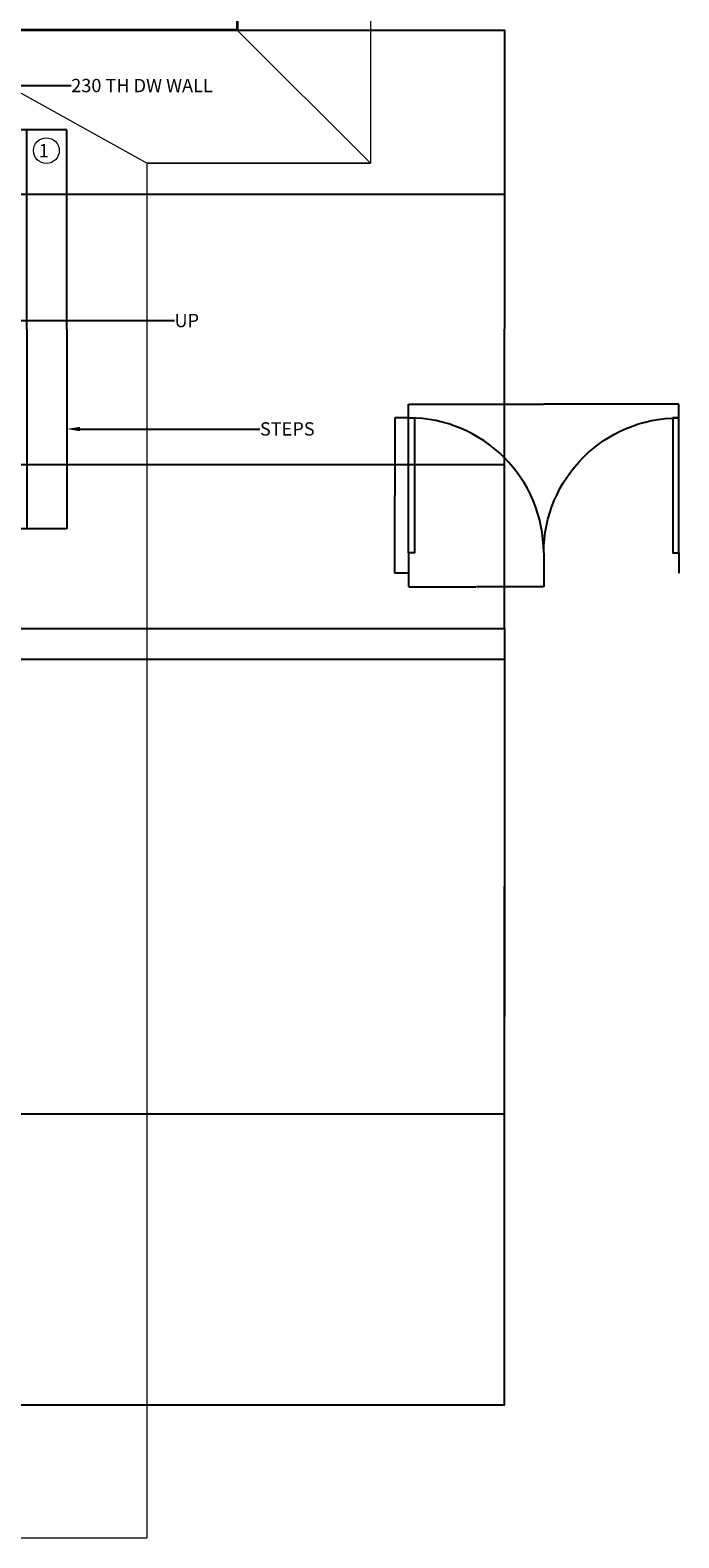
# Model space of a CAD drawing. Units: millimetres. Extents: x -8052 to 19968, y -37825 to -17505.
# Tile 9 of 10: x 10533 to 15409, y -36815 to -25475. Entities that reach past the tile are written whole.
import ezdxf
from ezdxf import colors
from ezdxf.entities.mleader import LeaderData, LeaderLine
from ezdxf.math import Vec2, Vec3

# ---------------------------------------------------------------- set-up
doc = ezdxf.new("R2010")
doc.units = ezdxf.units.MM
doc.header["$MEASUREMENT"] = 0
for name, color, linetype, lineweight in [('A-ANNO-DIMS', 2, 'Continuous', 18), ('A-ANNO-SYMB', 7, 'Continuous', 18), ('A-ANNO-TEXT', 7, 'Continuous', 18), ('A-DOOR', 3, 'Continuous', 25), ('A-FLOR', 8, 'Continuous', 18), ('A-FLOR-STRS', 7, 'Continuous', 25), ('A-WALL', 7, 'Continuous', 35)]:
    doc.layers.add(name, color=color, linetype=linetype, lineweight=lineweight)
doc.styles.get("Standard").update_dxf_attribs({"font": 'arial.ttf'})
doc.dimstyles.get("Standard").update_dxf_attribs({"dimtxt": 1.054, "dimasz": 1.055, "dimexe": 0.18, "dimexo": 0.0625, "dimgap": 0.09, "dimtad": 0, "dimtih": 1, "dimtoh": 1, "dimdec": 4, "dimzin": 0, "dimdsep": 46, "dimtxsty": 'Standard', "dimcen": 0.09, "dimadec": 0, "dimazin": 0, "dimtfac": 1, "dimtdec": 4, "dimtofl": 0, "dimtmove": 0, "dimatfit": 3, "dimfxl": 1, "dimtolj": 1, "dimtzin": 0, "dimarcsym": 0})

# ---------------------------------------------------------------- blocks, each defined once
blk = doc.blocks.new('*U21')
for p, q in [((0, 0), (0, -6)), ((40, 0), (40, -6))]:
    blk.add_line(p, q)
blk.add_lwpolyline([(0, 0), (0, 40), (1.75, 40), (1.75, 0)], close=True)
blk.add_arc((0, 0), 40, 0, 90)
blk = doc.blocks.new('STAIR-SIDE-ENTRY-3000')
for p, q in [((0, 1500), (0, 3000)), ((0, 3000), (1200, 3000)), ((300, 1500), (300, 3000)), ((300, 1500), (300, 3000)), ((600, 1500), (600, 3000)), ((900, 1500), (900, 3000)), ((0, 1500), (0, 1500)), ((0, 1500), (0, 0)), ((300, 1500), (300, 0)), ((600, 1500), (600, 0)), ((900, 1500), (900, 0)), ((0, 0), (1200, 0))]:
    blk.add_line(p, q)
blk = doc.blocks.new('*D97')
at = {"layer": 'A-ANNO-DIMS', "color": 0, "lineweight": -2, "transparency": 16777216}
for p, q in [((12090, -25475), (14100, -25475)), ((14099, -25476), (14099, -27724)), ((14099, -29974), (14099, -27725)), ((10410, -29975), (14100, -29975))]:
    blk.add_line(p, q, dxfattribs=at)
at = {"layer": 'A-ANNO-DIMS', "color": 0, "lineweight": 100, "transparency": 16777216}
for points in [[(14099, -25476), (14100, -25476), (14099, -25475)], [(14099, -29974), (14100, -29974), (14099, -29975)]]:
    blk.add_solid(points, dxfattribs=at)
at = {"layer": 'Defpoints', "color": 0, "lineweight": 100, "transparency": 16777216}
for p in [(12090, -25475), (10410, -29975), (14099, -29975)]:
    blk.add_point(p, dxfattribs=at)
at = {"layer": 'A-ANNO-DIMS', "color": 0, "transparency": 16777216, "insert": (14099, -27725), "char_height": 1.05, "attachment_point": 5}
blk.add_mtext('\\A1;4500', dxfattribs=at)
blk = doc.blocks.new('*D98')
at = {"layer": 'A-ANNO-DIMS', "color": 0, "lineweight": -2, "transparency": 16777216}
for p, q in [((10410, -29975), (14100, -29975)), ((14099, -29976), (14099, -32894)), ((14099, -35814), (14099, -32895)), ((10410, -35815), (14100, -35815))]:
    blk.add_line(p, q, dxfattribs=at)
at = {"layer": 'A-ANNO-DIMS', "color": 0, "lineweight": 100, "transparency": 16777216}
for points in [[(14099, -29976), (14100, -29976), (14099, -29975)], [(14099, -35814), (14100, -35814), (14099, -35815)]]:
    blk.add_solid(points, dxfattribs=at)
at = {"layer": 'Defpoints', "color": 0, "lineweight": 100, "transparency": 16777216}
for p in [(10410, -29975), (10410, -35815), (14099, -35815)]:
    blk.add_point(p, dxfattribs=at)
at = {"layer": 'A-ANNO-DIMS', "color": 0, "transparency": 16777216, "insert": (14099, -32895), "char_height": 1.05, "attachment_point": 5}
blk.add_mtext('\\A1;5840', dxfattribs=at)
blk = doc.blocks.new('*D109')
at = {"layer": 'A-ANNO-DIMS', "color": 0, "lineweight": -2, "transparency": 16777216}
for p, q in [((720, -30205), (14100, -30205)), ((14099, -30206), (14099, -31914)), ((14099, -33624), (14099, -31915)), ((950, -33625), (14100, -33625))]:
    blk.add_line(p, q, dxfattribs=at)
at = {"layer": 'A-ANNO-DIMS', "color": 0, "lineweight": 100, "transparency": 16777216}
for points in [[(14099, -30206), (14100, -30206), (14099, -30205)], [(14099, -33624), (14100, -33624), (14099, -33625)]]:
    blk.add_solid(points, dxfattribs=at)
at = {"layer": 'Defpoints', "color": 0, "lineweight": 100, "transparency": 16777216}
for p in [(720, -30205), (950, -33625), (14099, -33625)]:
    blk.add_point(p, dxfattribs=at)
at = {"layer": 'A-ANNO-DIMS', "color": 0, "transparency": 16777216, "insert": (14099, -31915), "char_height": 1.05, "attachment_point": 5}
blk.add_mtext('\\A1;3420', dxfattribs=at)
blk = doc.blocks.new('*D111')
at = {"layer": 'A-ANNO-DIMS', "color": 0, "lineweight": -2, "transparency": 16777216}
for p, q in [((-560, -26709), (14100, -26709)), ((14099, -26710), (14099, -27724)), ((14099, -28740), (14099, -27725)), ((-560, -28741), (14100, -28741))]:
    blk.add_line(p, q, dxfattribs=at)
at = {"layer": 'A-ANNO-DIMS', "color": 0, "lineweight": 100, "transparency": 16777216}
for points in [[(14099, -26710), (14100, -26710), (14099, -26709)], [(14099, -28740), (14100, -28740), (14099, -28741)]]:
    blk.add_solid(points, dxfattribs=at)
at = {"layer": 'Defpoints', "color": 0, "lineweight": 100, "transparency": 16777216}
for p in [(-560, -26709), (-560, -28741), (14099, -28741)]:
    blk.add_point(p, dxfattribs=at)
at = {"layer": 'A-ANNO-DIMS', "color": 0, "transparency": 16777216, "insert": (14099, -27725), "char_height": 1.05, "attachment_point": 5}
blk.add_mtext('\\A1;2032', dxfattribs=at)
blk = doc.blocks.new('*D126')
at = {"layer": 'A-ANNO-DIMS', "color": 0, "lineweight": -2, "transparency": 16777216}
for p, q in [((13377, -28391), (13377, -28288)), ((13378, -28289), (14391, -28289)), ((15408, -28289), (14395, -28289)), ((15409, -28391), (15409, -28288))]:
    blk.add_line(p, q, dxfattribs=at)
at = {"layer": 'A-ANNO-DIMS', "color": 0, "lineweight": 100, "transparency": 16777216}
for points in [[(13378, -28288), (13378, -28289), (13377, -28289)], [(15408, -28288), (15408, -28289), (15409, -28289)]]:
    blk.add_solid(points, dxfattribs=at)
at = {"layer": 'Defpoints', "color": 0, "lineweight": 100, "transparency": 16777216}
for p in [(15409, -28289), (13377, -28391), (15409, -28391)]:
    blk.add_point(p, dxfattribs=at)
at = {"layer": 'A-ANNO-DIMS', "color": 0, "transparency": 16777216, "insert": (14393, -28289), "char_height": 1.05, "attachment_point": 5}
blk.add_mtext('\\A1;2032', dxfattribs=at)
blk = doc.blocks.new('*D127')
at = {"layer": 'A-ANNO-DIMS', "color": 0, "lineweight": -2, "transparency": 16777216}
for p, q in [((13377, -28391), (13274, -28391)), ((13274, -28392), (13274, -28975)), ((13274, -29558), (13274, -28976)), ((13377, -29560), (13274, -29560))]:
    blk.add_line(p, q, dxfattribs=at)
at = {"layer": 'A-ANNO-DIMS', "color": 0, "lineweight": 100, "transparency": 16777216}
for points in [[(13274, -28392), (13275, -28392), (13274, -28391)], [(13274, -29558), (13275, -29558), (13274, -29560)]]:
    blk.add_solid(points, dxfattribs=at)
at = {"layer": 'Defpoints', "color": 0, "lineweight": 100, "transparency": 16777216}
for p in [(13274, -28391), (13377, -28391), (13377, -29560)]:
    blk.add_point(p, dxfattribs=at)
at = {"layer": 'A-ANNO-DIMS', "color": 0, "transparency": 16777216, "insert": (13274, -28975), "char_height": 1.05, "attachment_point": 5}
blk.add_mtext('\\A1;1168.4', dxfattribs=at)
blk = doc.blocks.new('*D128')
at = {"layer": 'A-ANNO-DIMS', "color": 0, "lineweight": -2, "transparency": 16777216}
for p, q in [((13377, -29407), (13377, -29662)), ((14393, -29407), (14393, -29662)), ((13378, -29662), (13883, -29662)), ((14392, -29662), (13887, -29662))]:
    blk.add_line(p, q, dxfattribs=at)
at = {"layer": 'A-ANNO-DIMS', "color": 0, "lineweight": 100, "transparency": 16777216}
for points in [[(13378, -29662), (13378, -29662), (13377, -29662)], [(14392, -29662), (14392, -29662), (14393, -29662)]]:
    blk.add_solid(points, dxfattribs=at)
at = {"layer": 'Defpoints', "color": 0, "lineweight": 100, "transparency": 16777216}
for p in [(13377, -29407), (14393, -29407), (14393, -29662)]:
    blk.add_point(p, dxfattribs=at)
at = {"layer": 'A-ANNO-DIMS', "color": 0, "transparency": 16777216, "insert": (13885, -29662), "char_height": 1.05, "attachment_point": 5}
blk.add_mtext('\\A1;1016', dxfattribs=at)

msp = doc.modelspace()

# ---------------------------------------------------------------- linework, layer by layer
at = {"layer": 'A-ANNO-SYMB'}
msp.add_circle((10654.35, -26381.051), 97, dxfattribs=at)
at = {"layer": 'A-FLOR'}
for p, q in [((13089.979, -18514.843), (13089.979, -26474.843)), ((11409.979, -26474.843), (9607.479, -25474.843)), ((12089.979, -25474.843), (13089.979, -26474.843)), ((11409.979, -26474.843), (11409.979, -36814.843)), ((13089.979, -26474.843), (11409.979, -26474.843)), ((13089.979, -26474.843), (11409.979, -26474.843)), ((11409.979, -26474.843), (13089.979, -26474.843)), ((11409.979, -26474.843), (11409.979, -36814.843)), ((-4710.021, -36814.843), (11409.979, -36814.843))]:
    msp.add_line(p, q, dxfattribs=at)
at = {"layer": 'A-WALL'}
for p, q in [((12089.979, -25244.843), (12089.979, -25474.843)), ((11859.979, -25474.843), (9359.979, -25474.843)), ((12089.979, -25474.843), (11859.979, -25474.843))]:
    msp.add_line(p, q, dxfattribs=at)

# ---------------------------------------------------------------- block references
at = {"layer": 'A-DOOR', "xscale": 25.39999999999996, "yscale": 25.39999999999996, "zscale": 25.39999999999996}
msp.add_blockref('*U21', (13376.928, -29407.126), dxfattribs=at)
at = {"layer": 'A-DOOR', "extrusion": (0, 0, -1), "xscale": 25.39999999999994, "yscale": 25.39999999999994, "zscale": -25.4}
msp.add_blockref('*U21', (-15408.928, -29407.126), dxfattribs=at)
at = {"layer": 'A-FLOR-STRS', "extrusion": (0, 0, -1), "zscale": -1}
msp.add_blockref('STAIR-SIDE-ENTRY-3000', (-10807.48, -29224.843), dxfattribs=at)

# ---------------------------------------------------------------- texts
at = {"layer": 'A-ANNO-TEXT', "insert": (10672.768, -26330.846), "char_height": 100, "attachment_point": 3}
msp.add_mtext_dynamic_manual_height_columns('1', width=159.07556, gutter_width=1, heights=[0], dxfattribs=at)

# ---------------------------------------------------------------- dimensions: what is measured, and where the dimension line sits
at = {"layer": 'A-ANNO-DIMS'}
for base, p1, p2, override, picture, middle in [((14099.479, -29974.843), (12089.979, -25474.843), (10409.979, -29974.843), {"dimdec": 0, "dimlfac": 1, "dimrnd": 0, "dimzin": 0, "dimdsep": 46, "dimlunit": 2}, '*D97', (14099.479, -27724.843)), ((14099.479, -28740.843), (-560.021, -26708.843), (-560.021, -28740.843), {"dimdec": 0, "dimlfac": 1, "dimrnd": 0, "dimzin": 0, "dimdsep": 46, "dimlunit": 2}, '*D111', (14099.479, -27724.843)), ((13274.428, -28391.126), (13376.928, -29559.526), (13376.928, -28391.126), {"dimdec": 1, "dimlfac": 1, "dimrnd": 0, "dimzin": 0, "dimdsep": 46, "dimlunit": 2}, '*D127', (13274.428, -28975.326)), ((14099.479, -35814.843), (10409.979, -29974.843), (10409.979, -35814.843), {"dimdec": 0, "dimlfac": 1, "dimrnd": 0, "dimzin": 0, "dimdsep": 46, "dimlunit": 2}, '*D98', (14099.479, -32894.843)), ((14099.479, -33624.843), (719.979, -30204.843), (949.979, -33624.843), {"dimdec": 0, "dimlfac": 1, "dimrnd": 0, "dimzin": 0, "dimdsep": 46, "dimlunit": 2}, '*D109', (14099.479, -31914.843))]:
    dim = msp.add_linear_dim(base=base, p1=p1, p2=p2, angle=90, dimstyle='Standard', override=override, dxfattribs=at)
    dim.commit()
    dim.dimension.update_dxf_attribs({"geometry": picture, "text_midpoint": middle})
for base, p1, p2, picture, middle in [((15408.928, -28288.626), (13376.928, -28391.126), (15408.928, -28391.126), '*D126', (14392.928, -28288.626)), ((14392.928, -29662.026), (13376.928, -29407.126), (14392.928, -29407.126), '*D128', (13884.928, -29662.026))]:
    dim = msp.add_linear_dim(base=base, p1=p1, p2=p2, dimstyle='Standard', override={"dimdec": 0, "dimlfac": 1, "dimrnd": 0, "dimzin": 0, "dimdsep": 46, "dimlunit": 2}, dxfattribs=at)
    dim.commit()
    dim.dimension.update_dxf_attribs({"geometry": picture, "text_midpoint": middle})

# ---------------------------------------------------------------- leaders
at = {"layer": 'A-ANNO-TEXT'}
ml = msp.add_multileader_mtext('Standard', dxfattribs=at)
ml.set_content('230 TH DW WALL', color=256)
ml.set_leader_properties()
ml.build(insert=Vec2(0, 0))
ml.multileader.update_dxf_attribs({"dogleg_length": 0.36, "arrow_head_size": 150})
ctx = ml.context
ctx.base_point, ctx.char_height, ctx.arrow_head_size, ctx.landing_gap_size, ctx.plane_origin = Vec3(10841.096, -25892.244), 100, 150, 0.09, Vec3(9482.701, -25892.244)
notes = []
notes.append((ctx, [(0, (1, 1, 0), (10840.736, -25892.244), (1, 0), 0.36, [(0, [(9482.701, -25892.244)], 0, [])])]))
ctx.mtext.insert, ctx.mtext.flow_direction = Vec3(10841.186, -25841.357), 5
ml = msp.add_multileader_mtext('Standard', dxfattribs=at)
ml.set_content('\\pxt1;UP', color=256)
ml.set_leader_properties()
ml.build(insert=Vec2(0, 0))
ml.multileader.update_dxf_attribs({"dogleg_length": 0.36, "arrow_head_size": 100})
ctx = ml.context
ctx.base_point, ctx.char_height, ctx.arrow_head_size, ctx.landing_gap_size, ctx.plane_origin = Vec3(11617.533, -27659.789), 100, 100, 0.09, Vec3(10207.479, -27659.789)
notes.append((ctx, [(0, (1, 1, 0), (11617.173, -27659.789), (1, 0), 0.36, [(0, [(10207.479, -27659.789)], 0, [])])]))
ctx.mtext.insert, ctx.mtext.width, ctx.mtext.flow_direction = Vec3(11617.623, -27608.937), 0.34019, 5
ml = msp.add_multileader_mtext('Standard', dxfattribs=at)
ml.set_content('STEPS', color=256)
ml.set_leader_properties()
ml.build(insert=Vec2(0, 0))
ml.multileader.update_dxf_attribs({"dogleg_length": 0.36, "arrow_head_size": 100})
ctx = ml.context
ctx.base_point, ctx.char_height, ctx.arrow_head_size, ctx.landing_gap_size, ctx.plane_origin = Vec3(12260, -28474.843), 100, 100, 0.09, Vec3(10807.479, -28474.843)
notes.append((ctx, [(0, (1, 1, 0), (12259.64, -28474.843), (1, 0), 0.36, [(0, [(10807.479, -28474.843)], 0, [])])]))
ctx.mtext.insert, ctx.mtext.flow_direction = Vec3(12260.09, -28423.99), 5
for ctx, leaders in notes:
    for number, flags, end, landing, length, lines in leaders:
        leader = LeaderData()
        leader.index, (leader.has_last_leader_line, leader.has_dogleg_vector, leader.attachment_direction) = number, flags
        leader.last_leader_point, leader.dogleg_vector, leader.dogleg_length = Vec3(end), Vec3(landing), length
        for number, points, colour, breaks in lines:
            line = LeaderLine()
            line.index, line.vertices, line.color, line.breaks = number, Vec3.list(points), colors.encode_raw_color(colour), breaks
            leader.lines.append(line)
        ctx.leaders.append(leader)

doc.saveas('drawing.dxf')
